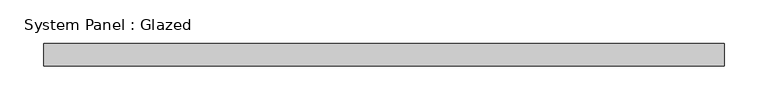
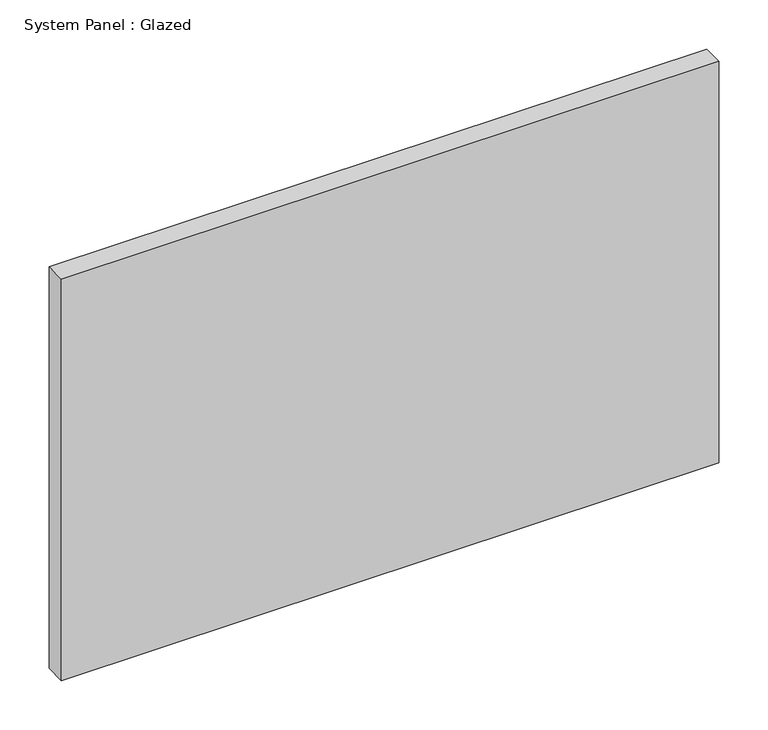
"""IFC4 building model written with IfcOpenShell, lengths in millimetres: plate geometry, System Panel : Glazed."""

from ifc_helpers import new_model, si_unit, origin, origin_with_axes, place, context, project, spatial, polyline, outline, extrude, source, transform, mapped, element, save


def system_panel_glazed_55b634e8(model_context):
    return source(origin(), model_context, "Body", "SweptSolid", [
        extrude(outline(polyline([(387.35, 19.05), (-387.35, 19.05), (-387.35, 44.45), (387.35, 44.45), (387.35, 19.05)])), origin_with_axes(), (0.0, 0.0, 1.0), 500.0403046),
    ])


if __name__ == "__main__":
    model = new_model("IFC4")
    model_context = context("Model", 3, world=origin())
    ifc_project = project(units=[si_unit("LENGTHUNIT", "METRE", prefix="MILLI")], contexts=[model_context])
    site = spatial("IfcSite", under=ifc_project)
    building = spatial("IfcBuilding", under=site)
    placement = place(None, origin())
    system_panel_glazed_shape = system_panel_glazed_55b634e8(model_context)
    element("IfcPlate", 1, ObjectType="System Panel : Glazed", at=placement, inside=building, context=model_context, shape_type="MappedRepresentation", body=[
        mapped(system_panel_glazed_shape, transform((0.0, 0.0, 0.0), x_axis=(1.0, 0.0, 0.0), y_axis=(0.0, 1.0, 0.0), z_axis=(0.0, 0.0, 1.0))),
    ])
    save(model, "model.ifc")

# Revit data of these elements
# Type "System Panel : Glazed"
#   Construction Type Id = "GSP4R"
#   Analytic Construction = "1/8 in Pilkington single glazing"
#   Visual Light Transmittance = 0.9
#   Solar Heat Gain Coefficient = 0.86
#   Heat Transfer Coefficient (U) = 1.18115 BTU/(h·ft²·°F)
#   Define Thermal Properties by = 1
# Element 1 (IfcPlate, "System Panel : Glazed")
#   Materials on its faces: "Glass"
# Materials
#   "Glass": class "Glass", colour RGB 0 128 192, transparency 0.75, Description = "Soda Lime Glass", Cost = 0
